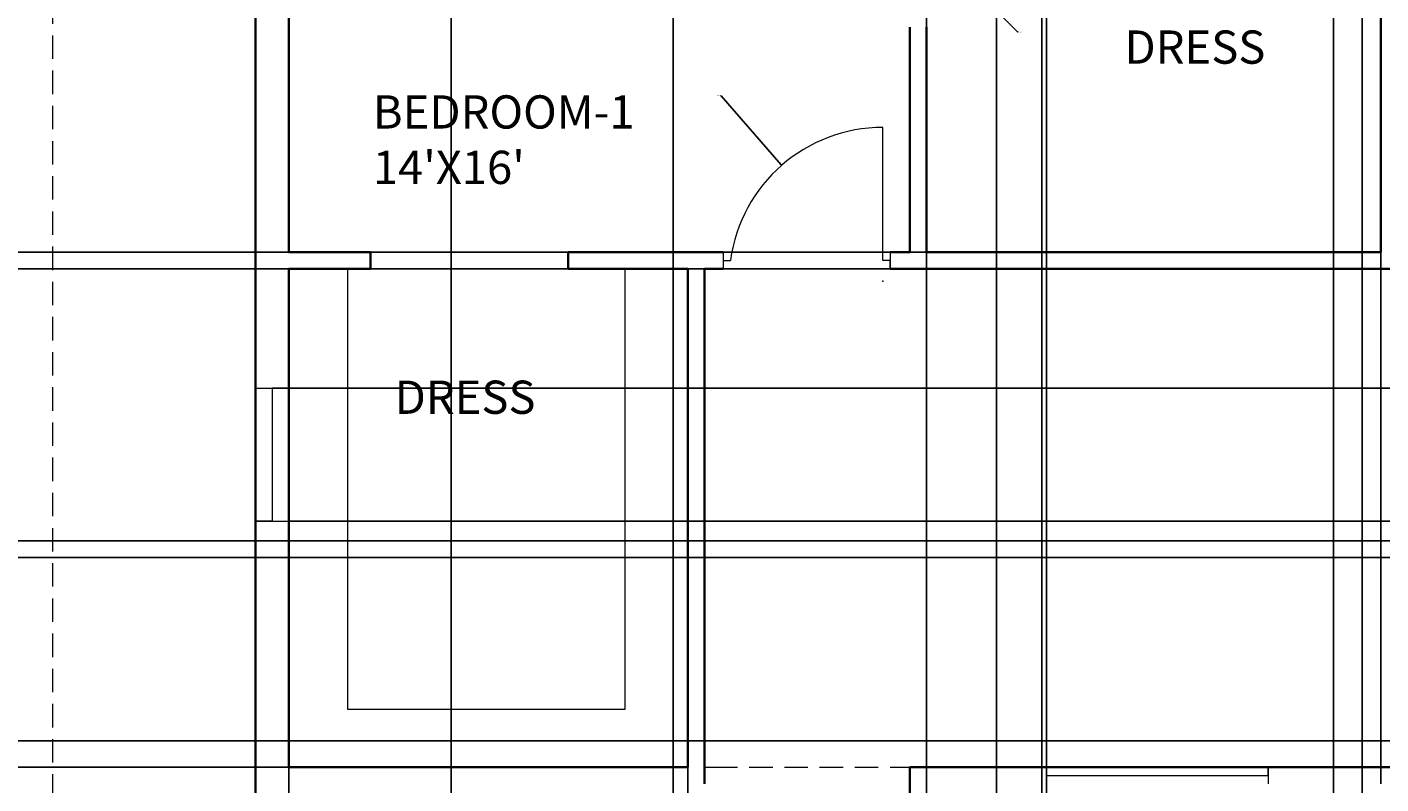
# Model space of a CAD drawing. Units: inches. Extents: x 1770 to 2988, y 1161 to 3221.
# Tile 11 of 44: x 2090 to 2456, y 2032 to 2237. Entities that reach past the tile are written whole.
import ezdxf

# ---------------------------------------------------------------- set-up
doc = ezdxf.new("R2010")
doc.units = ezdxf.units.IN
doc.linetypes.add('DASHED2', pattern=[9.525, 6.35, -3.175])
for name, color, linetype, lineweight in [('A-ANNO-DIMS', 2, 'Continuous', 18), ('A-AREA-IDEN', 7, 'Continuous', 18), ('A-DOOR', 4, 'Continuous', 18), ('A-FLOR-CASE', 8, 'Continuous', 18), ('A-GLAZ', 4, 'Continuous', 18), ('A-ROOF-OVHD', 7, 'DASHED2', 18), ('A-WALL', 7, 'Continuous', 35), ('A-WALL-OVHD', 7, 'DASHED2', 18)]:
    doc.layers.add(name, color=color, linetype=linetype, lineweight=lineweight)
doc.styles.get("Standard").update_dxf_attribs({"font": 'arial.ttf'})
doc.dimstyles.get("Standard").update_dxf_attribs({"dimtxt": 0.18, "dimasz": 0.18, "dimexe": 0.18, "dimexo": 0.0625, "dimgap": 0.09, "dimtad": 0, "dimtih": 1, "dimtoh": 1, "dimdec": 4, "dimzin": 0, "dimdsep": 46, "dimtxsty": 'Standard', "dimcen": 0.09, "dimadec": 0, "dimazin": 0, "dimtfac": 1, "dimtdec": 4, "dimtofl": 0, "dimtmove": 0, "dimatfit": 3, "dimfxl": 1, "dimtolj": 1, "dimtzin": 0, "dimarcsym": 0})

# ---------------------------------------------------------------- blocks, each defined once
blk = doc.blocks.new('WIN-60-COURTYARD')
for p, q in [((0, 4.5), (0, 0)), ((60, 2.25), (60, 4.5)), ((60, 4.5), (60, 0)), ((0, 0), (0, 2.25)), ((0, 2.25), (60, 2.25))]:
    blk.add_line(p, q)
blk = doc.blocks.new('*D63')
at = {"layer": 'A-ANNO-DIMS', "color": 0, "lineweight": -2, "transparency": 16777216}
for p, q in [((2352.17, 1323.59), (2352.17, 2570.7)), ((2352.35, 2570.52), (2401.24, 2570.52)), ((2450.91, 2570.52), (2402.02, 2570.52)), ((2451.09, 1323.59), (2451.09, 2570.7))]:
    blk.add_line(p, q, dxfattribs=at)
at = {"layer": 'A-ANNO-DIMS', "color": 0, "transparency": 16777216}
for points in [[(2352.35, 2570.55), (2352.35, 2570.49), (2352.17, 2570.52)], [(2450.91, 2570.55), (2450.91, 2570.49), (2451.09, 2570.52)]]:
    blk.add_solid(points, dxfattribs=at)
at = {"layer": 'Defpoints', "color": 0, "transparency": 16777216}
for p in [(2451.09, 2570.52), (2352.17, 1323.53), (2451.09, 1323.53)]:
    blk.add_point(p, dxfattribs=at)
at = {"layer": 'A-ANNO-DIMS', "color": 0, "transparency": 16777216, "insert": (2401.63, 2570.52), "char_height": 0.18, "attachment_point": 5}
blk.add_mtext('\\A1;98.93', dxfattribs=at)
blk = doc.blocks.new('*D68')
at = {"layer": 'A-ANNO-DIMS', "color": 0, "lineweight": -2, "transparency": 16777216}
for p, q in [((2333.2, 2031.76), (2333.2, 2570.7)), ((2333.38, 2570.52), (2394.42, 2570.52)), ((2456.02, 2570.52), (2394.98, 2570.52)), ((2456.2, 2031.76), (2456.2, 2570.7))]:
    blk.add_line(p, q, dxfattribs=at)
at = {"layer": 'A-ANNO-DIMS', "color": 0, "transparency": 16777216}
for points in [[(2333.38, 2570.55), (2333.38, 2570.49), (2333.2, 2570.52)], [(2456.02, 2570.55), (2456.02, 2570.49), (2456.2, 2570.52)]]:
    blk.add_solid(points, dxfattribs=at)
at = {"layer": 'Defpoints', "color": 0, "transparency": 16777216}
for p in [(2456.2, 2570.52), (2333.2, 2031.7), (2456.2, 2031.7)]:
    blk.add_point(p, dxfattribs=at)
at = {"layer": 'A-ANNO-DIMS', "color": 0, "transparency": 16777216, "insert": (2394.7, 2570.52), "char_height": 0.18, "attachment_point": 5}
blk.add_mtext('\\A1;123', dxfattribs=at)
blk = doc.blocks.new('*D70')
at = {"layer": 'A-ANNO-DIMS', "color": 0, "lineweight": -2, "transparency": 16777216}
for p, q in [((2160.7, 2171.14), (2160.7, 1165.57)), ((2268.7, 2171.14), (2268.7, 1165.57)), ((2160.88, 1165.75), (2214.42, 1165.75)), ((2268.52, 1165.75), (2214.98, 1165.75))]:
    blk.add_line(p, q, dxfattribs=at)
at = {"layer": 'A-ANNO-DIMS', "color": 0, "transparency": 16777216}
for points in [[(2160.88, 1165.78), (2160.88, 1165.72), (2160.7, 1165.75)], [(2268.52, 1165.78), (2268.52, 1165.72), (2268.7, 1165.75)]]:
    blk.add_solid(points, dxfattribs=at)
at = {"layer": 'Defpoints', "color": 0, "transparency": 16777216}
for p in [(2160.7, 2171.2), (2268.7, 2171.2), (2268.7, 1165.75)]:
    blk.add_point(p, dxfattribs=at)
at = {"layer": 'A-ANNO-DIMS', "color": 0, "transparency": 16777216, "insert": (2214.7, 1165.75), "char_height": 0.18, "attachment_point": 5}
blk.add_mtext('\\A1;108', dxfattribs=at)
blk = doc.blocks.new('*D71')
at = {"layer": 'A-ANNO-DIMS', "color": 0, "lineweight": -2, "transparency": 16777216}
for p, q in [((2160.63, 2171.2), (1907.1, 2171.2)), ((1907.28, 2171.02), (1907.28, 2103.88)), ((1907.28, 2036.38), (1907.28, 2103.52)), ((2160.63, 2036.2), (1907.1, 2036.2))]:
    blk.add_line(p, q, dxfattribs=at)
at = {"layer": 'A-ANNO-DIMS', "color": 0, "transparency": 16777216}
for points in [[(1907.25, 2171.02), (1907.31, 2171.02), (1907.28, 2171.2)], [(1907.25, 2036.38), (1907.31, 2036.38), (1907.28, 2036.2)]]:
    blk.add_solid(points, dxfattribs=at)
at = {"layer": 'Defpoints', "color": 0, "transparency": 16777216}
for p in [(2160.7, 2171.2), (1907.28, 2036.2), (2160.7, 2036.2)]:
    blk.add_point(p, dxfattribs=at)
at = {"layer": 'A-ANNO-DIMS', "color": 0, "transparency": 16777216, "insert": (1907.28, 2103.7), "char_height": 0.18, "attachment_point": 5}
blk.add_mtext('\\A1;135', dxfattribs=at)
blk = doc.blocks.new('*D72')
at = {"layer": 'A-ANNO-DIMS', "color": 0, "lineweight": -2, "transparency": 16777216}
for p, q in [((2456.13, 2267.2), (1907.1, 2267.2)), ((1907.28, 2267.02), (1907.28, 2221.63)), ((1907.28, 2175.88), (1907.28, 2221.27)), ((2456.13, 2175.7), (1907.1, 2175.7))]:
    blk.add_line(p, q, dxfattribs=at)
at = {"layer": 'A-ANNO-DIMS', "color": 0, "transparency": 16777216}
for points in [[(1907.25, 2267.02), (1907.31, 2267.02), (1907.28, 2267.2)], [(1907.25, 2175.88), (1907.31, 2175.88), (1907.28, 2175.7)]]:
    blk.add_solid(points, dxfattribs=at)
at = {"layer": 'Defpoints', "color": 0, "transparency": 16777216}
for p in [(1907.28, 2267.2), (2456.2, 2267.2), (2456.2, 2175.7)]:
    blk.add_point(p, dxfattribs=at)
at = {"layer": 'A-ANNO-DIMS', "color": 0, "transparency": 16777216, "insert": (1907.28, 2221.45), "char_height": 0.18, "attachment_point": 5}
blk.add_mtext('\\A1;91.5', dxfattribs=at)
blk = doc.blocks.new('*D75')
at = {"layer": 'A-ANNO-DIMS', "color": 0, "lineweight": -2, "transparency": 16777216}
for p, q in [((2523.36, 2171.2), (1907.1, 2171.2)), ((1907.28, 2171.02), (1907.28, 2134.56)), ((1907.28, 2097.72), (1907.28, 2134.19)), ((2523.36, 2097.54), (1907.1, 2097.54))]:
    blk.add_line(p, q, dxfattribs=at)
at = {"layer": 'A-ANNO-DIMS', "color": 0, "transparency": 16777216}
for points in [[(1907.25, 2171.02), (1907.31, 2171.02), (1907.28, 2171.2)], [(1907.25, 2097.72), (1907.31, 2097.72), (1907.28, 2097.54)]]:
    blk.add_solid(points, dxfattribs=at)
at = {"layer": 'Defpoints', "color": 0, "transparency": 16777216}
for p in [(2523.42, 2171.2), (1907.28, 2097.54), (2523.42, 2097.54)]:
    blk.add_point(p, dxfattribs=at)
at = {"layer": 'A-ANNO-DIMS', "color": 0, "transparency": 16777216, "insert": (1907.28, 2134.37), "char_height": 0.18, "attachment_point": 5}
blk.add_mtext('\\A1;73.66', dxfattribs=at)
blk = doc.blocks.new('*D79')
at = {"layer": 'A-ANNO-DIMS', "color": 0, "lineweight": -2, "transparency": 16777216}
for p, q in [((2151.7, 1610.26), (2151.7, 2570.7)), ((2151.88, 2570.52), (2177.78, 2570.52)), ((2204.48, 2570.52), (2178.57, 2570.52)), ((2204.66, 1610.26), (2204.66, 2570.7))]:
    blk.add_line(p, q, dxfattribs=at)
at = {"layer": 'A-ANNO-DIMS', "color": 0, "transparency": 16777216}
for points in [[(2151.88, 2570.55), (2151.88, 2570.49), (2151.7, 2570.52)], [(2204.48, 2570.55), (2204.48, 2570.49), (2204.66, 2570.52)]]:
    blk.add_solid(points, dxfattribs=at)
at = {"layer": 'Defpoints', "color": 0, "transparency": 16777216}
for p in [(2204.66, 2570.52), (2151.7, 1610.2), (2204.66, 1610.2)]:
    blk.add_point(p, dxfattribs=at)
at = {"layer": 'A-ANNO-DIMS', "color": 0, "transparency": 16777216, "insert": (2178.18, 2570.52), "char_height": 0.18, "attachment_point": 5}
blk.add_mtext('\\A1;52.96', dxfattribs=at)
blk = doc.blocks.new('*D80')
at = {"layer": 'A-ANNO-DIMS', "color": 0, "lineweight": -2, "transparency": 16777216}
for p, q in [((2264.66, 1610.26), (2264.66, 2570.7)), ((2264.84, 2570.52), (2314.14, 2570.52)), ((2364.23, 2570.52), (2314.93, 2570.52)), ((2364.41, 1610.26), (2364.41, 2570.7))]:
    blk.add_line(p, q, dxfattribs=at)
at = {"layer": 'A-ANNO-DIMS', "color": 0, "transparency": 16777216}
for points in [[(2264.84, 2570.55), (2264.84, 2570.49), (2264.66, 2570.52)], [(2364.23, 2570.55), (2364.23, 2570.49), (2364.41, 2570.52)]]:
    blk.add_solid(points, dxfattribs=at)
at = {"layer": 'Defpoints', "color": 0, "transparency": 16777216}
for p in [(2364.41, 2570.52), (2264.66, 1610.2), (2364.41, 1610.2)]:
    blk.add_point(p, dxfattribs=at)
at = {"layer": 'A-ANNO-DIMS', "color": 0, "transparency": 16777216, "insert": (2314.53, 2570.52), "char_height": 0.18, "attachment_point": 5}
blk.add_mtext('\\A1;99.76', dxfattribs=at)
blk = doc.blocks.new('*D81')
at = {"layer": 'A-ANNO-DIMS', "color": 0, "lineweight": -2, "transparency": 16777216}
for p, q in [((2364.41, 1610.26), (2364.41, 2570.7)), ((2364.59, 2570.52), (2403.51, 2570.52)), ((2443.21, 2570.52), (2404.29, 2570.52)), ((2443.39, 1610.26), (2443.39, 2570.7))]:
    blk.add_line(p, q, dxfattribs=at)
at = {"layer": 'A-ANNO-DIMS', "color": 0, "transparency": 16777216}
for points in [[(2364.59, 2570.55), (2364.59, 2570.49), (2364.41, 2570.52)], [(2443.21, 2570.55), (2443.21, 2570.49), (2443.39, 2570.52)]]:
    blk.add_solid(points, dxfattribs=at)
at = {"layer": 'Defpoints', "color": 0, "transparency": 16777216}
for p in [(2443.39, 2570.52), (2364.41, 1610.2), (2443.39, 1610.2)]:
    blk.add_point(p, dxfattribs=at)
at = {"layer": 'A-ANNO-DIMS', "color": 0, "transparency": 16777216, "insert": (2403.9, 2570.52), "char_height": 0.18, "attachment_point": 5}
blk.add_mtext('\\A1;78.97', dxfattribs=at)
blk = doc.blocks.new('*D82')
at = {"layer": 'A-ANNO-DIMS', "color": 0, "lineweight": -2, "transparency": 16777216}
for p, q in [((2443.39, 1610.26), (2443.39, 2570.7)), ((2443.57, 2570.52), (2486.45, 2570.52)), ((2530.12, 2570.52), (2487.24, 2570.52)), ((2530.3, 1610.26), (2530.3, 2570.7))]:
    blk.add_line(p, q, dxfattribs=at)
at = {"layer": 'A-ANNO-DIMS', "color": 0, "transparency": 16777216}
for points in [[(2443.57, 2570.55), (2443.57, 2570.49), (2443.39, 2570.52)], [(2530.12, 2570.55), (2530.12, 2570.49), (2530.3, 2570.52)]]:
    blk.add_solid(points, dxfattribs=at)
at = {"layer": 'Defpoints', "color": 0, "transparency": 16777216}
for p in [(2530.3, 2570.52), (2443.39, 1610.2), (2530.3, 1610.2)]:
    blk.add_point(p, dxfattribs=at)
at = {"layer": 'A-ANNO-DIMS', "color": 0, "transparency": 16777216, "insert": (2486.85, 2570.52), "char_height": 0.18, "attachment_point": 5}
blk.add_mtext('\\A1;86.92', dxfattribs=at)
blk = doc.blocks.new('*D88')
at = {"layer": 'A-ANNO-DIMS', "color": 0, "lineweight": -2, "transparency": 16777216}
for p, q in [((2523.36, 2093.04), (1907.1, 2093.04)), ((1907.28, 2092.86), (1907.28, 2068.4)), ((1907.28, 2043.57), (1907.28, 2068.04)), ((2523.36, 2043.39), (1907.1, 2043.39))]:
    blk.add_line(p, q, dxfattribs=at)
at = {"layer": 'A-ANNO-DIMS', "color": 0, "transparency": 16777216}
for points in [[(1907.25, 2092.86), (1907.31, 2092.86), (1907.28, 2093.04)], [(1907.25, 2043.57), (1907.31, 2043.57), (1907.28, 2043.39)]]:
    blk.add_solid(points, dxfattribs=at)
at = {"layer": 'Defpoints', "color": 0, "transparency": 16777216}
for p in [(1907.28, 2093.04), (2523.42, 2093.04), (2523.42, 2043.39)]:
    blk.add_point(p, dxfattribs=at)
at = {"layer": 'A-ANNO-DIMS', "color": 0, "transparency": 16777216, "insert": (1907.28, 2068.22), "char_height": 0.18, "attachment_point": 5}
blk.add_mtext('\\A1;49.65', dxfattribs=at)
blk = doc.blocks.new('*D89')
at = {"layer": 'A-ANNO-DIMS', "color": 0, "lineweight": -2, "transparency": 16777216}
for p, q in [((2160.76, 2138.84), (2866.87, 2138.84)), ((2866.69, 2138.66), (2866.69, 2121.02)), ((2866.69, 2103.02), (2866.69, 2120.66)), ((2160.76, 2102.84), (2866.87, 2102.84))]:
    blk.add_line(p, q, dxfattribs=at)
at = {"layer": 'A-ANNO-DIMS', "color": 0, "transparency": 16777216}
for points in [[(2866.66, 2138.66), (2866.72, 2138.66), (2866.69, 2138.84)], [(2866.66, 2103.02), (2866.72, 2103.02), (2866.69, 2102.84)]]:
    blk.add_solid(points, dxfattribs=at)
at = {"layer": 'Defpoints', "color": 0, "transparency": 16777216}
for p in [(2160.7, 2138.84), (2866.69, 2138.84), (2160.7, 2102.84)]:
    blk.add_point(p, dxfattribs=at)
at = {"layer": 'A-ANNO-DIMS', "color": 0, "transparency": 16777216, "insert": (2866.69, 2120.84), "char_height": 0.18, "attachment_point": 5}
blk.add_mtext('\\A1;36', dxfattribs=at)
blk = doc.blocks.new('*D91')
at = {"layer": 'A-ANNO-DIMS', "color": 0, "lineweight": -2, "transparency": 16777216}
for p, q in [((2333.2, 1839.76), (2333.2, 2570.7)), ((2333.38, 2570.52), (2348.97, 2570.52)), ((2365.49, 2570.52), (2349.9, 2570.52)), ((2365.67, 1839.76), (2365.67, 2570.7))]:
    blk.add_line(p, q, dxfattribs=at)
at = {"layer": 'A-ANNO-DIMS', "color": 0, "transparency": 16777216}
for points in [[(2333.38, 2570.55), (2333.38, 2570.49), (2333.2, 2570.52)], [(2365.49, 2570.55), (2365.49, 2570.49), (2365.67, 2570.52)]]:
    blk.add_solid(points, dxfattribs=at)
at = {"layer": 'Defpoints', "color": 0, "transparency": 16777216}
for p in [(2365.67, 2570.52), (2333.2, 1839.7), (2365.67, 1839.7)]:
    blk.add_point(p, dxfattribs=at)
at = {"layer": 'A-ANNO-DIMS', "color": 0, "transparency": 16777216, "insert": (2349.43, 2570.52), "char_height": 0.18, "attachment_point": 5}
blk.add_mtext('\\A1;32.476', dxfattribs=at)
blk = doc.blocks.new('*D110')
at = {"layer": 'A-ANNO-DIMS', "color": 0, "lineweight": -2, "transparency": 16777216}
for p, q in [((2277.46, 2218.01), (2277.64, 2218.01)), ((2277.64, 2218.01), (2293.95, 2199.32)), ((2321.35, 2167.81), (2321.53, 2167.81)), ((2321.44, 2167.72), (2321.44, 2167.9))]:
    blk.add_line(p, q, dxfattribs=at)
at = {"layer": 'A-ANNO-DIMS', "color": 0, "transparency": 16777216}
blk.add_solid([(2293.97, 2199.34), (2293.92, 2199.3), (2294.06, 2199.19)], dxfattribs=at)
at = {"layer": 'Defpoints', "color": 0, "transparency": 16777216}
for p in [(2294.06, 2199.19), (2321.44, 2167.81)]:
    blk.add_point(p, dxfattribs=at)
at = {"layer": 'A-ANNO-DIMS', "color": 0, "transparency": 16777216, "insert": (2276.98, 2218.01), "char_height": 0.18, "attachment_point": 5}
blk.add_mtext('\\A1;R41.64', dxfattribs=at)
blk = doc.blocks.new('*D112')
at = {"layer": 'A-ANNO-DIMS', "color": 0, "lineweight": -2, "transparency": 16777216}
for p, q in [((2331.23, 2262.24), (2331.41, 2262.24)), ((2331.32, 2262.15), (2331.32, 2262.33)), ((2357.84, 2235.3), (2348.02, 2245.28)), ((2358.02, 2235.3), (2357.84, 2235.3))]:
    blk.add_line(p, q, dxfattribs=at)
at = {"layer": 'A-ANNO-DIMS', "color": 0, "transparency": 16777216}
blk.add_solid([(2348.04, 2245.3), (2348, 2245.26), (2347.89, 2245.41)], dxfattribs=at)
at = {"layer": 'Defpoints', "color": 0, "transparency": 16777216}
for p in [(2331.32, 2262.24), (2347.89, 2245.41)]:
    blk.add_point(p, dxfattribs=at)
at = {"layer": 'A-ANNO-DIMS', "color": 0, "transparency": 16777216, "insert": (2358.5, 2235.3), "char_height": 0.18, "attachment_point": 5}
blk.add_mtext('\\A1;R23.63', dxfattribs=at)

msp = doc.modelspace()

# ---------------------------------------------------------------- linework, layer by layer
at = {"layer": 'A-DOOR'}
for p, q in [((2321.4422, 2173.4521), (2321.4422, 2209.4521)), ((2278.1834, 2175.7021), (2278.1834, 2171.2021)), ((2278.1834, 2173.4521), (2280.1834, 2173.4521)), ((2323.4422, 2173.4521), (2321.4422, 2173.4521)), ((2323.4422, 2175.7021), (2323.4422, 2171.2021)), ((2323.4422, 2171.2021), (2323.4422, 2173.4521))]:
    msp.add_line(p, q, dxfattribs=at)
msp.add_arc((2321.4422, 2167.8092), 41.6429, 90, 172.212025, dxfattribs=at)
at = {"layer": 'A-FLOR-CASE'}
for p, q in [((2176.5309, 2171.2021), (2176.5309, 2051.9256)), ((2251.7333, 2051.9256), (2251.7333, 2171.2021)), ((2176.5309, 2051.9256), (2251.7333, 2051.9256))]:
    msp.add_line(p, q, dxfattribs=at)
at = {"layer": 'A-GLAZ'}
for p, q in [((2151.696, 2138.8392), (2160.696, 2138.8392)), ((2160.696, 2138.8392), (2156.196, 2138.8392)), ((2156.196, 2138.8392), (2156.196, 2102.8392)), ((2156.196, 2102.8392), (2151.696, 2102.8392)), ((2151.696, 2102.8392), (2160.696, 2102.8392))]:
    msp.add_line(p, q, dxfattribs=at)
at = {"layer": 'A-ROOF-OVHD'}
msp.add_line((2096.7313, 2405.7876), (2096.7313, 1610.2021), dxfattribs=at)
at = {"layer": 'A-WALL'}
for p, q in [((2151.696, 2376.7021), (2151.696, 1610.2021)), ((2160.696, 2367.7021), (2160.696, 2175.7021)), ((2456.196, 2267.2021), (2456.196, 2175.7021)), ((2328.696, 2236.6179), (2328.696, 2175.7021)), ((2333.196, 2236.6179), (2333.196, 2175.7021)), ((2160.696, 2175.7021), (2182.7786, 2175.7021)), ((2182.7786, 2175.7021), (2182.7786, 2171.2021)), ((2236.2643, 2175.7021), (2236.2643, 2171.2021)), ((2236.2643, 2175.7021), (2278.1834, 2175.7021)), ((2323.4422, 2175.7021), (2328.696, 2175.7021)), ((2333.196, 2175.7021), (2456.196, 2175.7021)), ((2160.696, 2171.2021), (2182.7786, 2171.2021)), ((2160.696, 2171.2021), (2160.696, 2036.2021)), ((2236.2643, 2171.2021), (2268.696, 2171.2021)), ((2268.696, 2171.2021), (2268.696, 2036.2021)), ((2273.196, 2171.2021), (2273.196, 2031.7021)), ((2273.196, 2171.2021), (2278.1834, 2171.2021)), ((2323.4422, 2171.2021), (2468.7272, 2171.2021)), ((2160.696, 2036.2021), (2268.696, 2036.2021)), ((2328.696, 2036.2021), (2328.696, 1835.2021)), ((2328.696, 2036.2021), (2460.696, 2036.2021))]:
    msp.add_line(p, q, dxfattribs=at)
at = {"layer": 'A-WALL-OVHD'}
for p, q in [((2184.4959, 2175.7021), (2236.2643, 2175.7021)), ((2236.2643, 2171.2021), (2182.7786, 2171.2021)), ((2273.196, 2036.2021), (2275.7476, 2036.2021)), ((2275.7476, 2036.2021), (2328.696, 2036.2021))]:
    msp.add_line(p, q, dxfattribs=at)

# ---------------------------------------------------------------- block references
at = {"layer": 'A-GLAZ'}
msp.add_blockref('WIN-60-COURTYARD', (2365.672, 2031.702), dxfattribs=at)

# ---------------------------------------------------------------- texts
at = {"layer": 'A-AREA-IDEN', "char_height": 9, "attachment_point": 1}
for s, width, insert in [('DRESS', 37.691321, (2386.8048, 2235.6986)), ("BEDROOM-1\\P14'X16'", 127.484882, (2183.43, 2218.1375)), ('DRESS', 67.187897, (2189.3188, 2140.8976))]:
    msp.add_mtext_dynamic_manual_height_columns(s, width=width, gutter_width=12.5, heights=[0], dxfattribs=dict(at, insert=insert))

# ---------------------------------------------------------------- dimensions: what is measured, and where the dimension line sits
at = {"layer": 'A-ANNO-DIMS'}
for base, p1, p2, override, picture, middle in [((2204.6568, 2570.5247), (2151.696, 1610.2021), (2204.6568, 1610.2021), {"dimdec": 2, "dimlfac": 1, "dimrnd": 0, "dimzin": 0, "dimdsep": 46, "dimlunit": 2}, '*D79', (2178.1764, 2570.5247)), ((2364.4122, 2570.5247), (2264.6568, 1610.2021), (2364.4122, 1610.2021), {"dimdec": 2, "dimlfac": 1, "dimrnd": 0, "dimzin": 0, "dimdsep": 46, "dimlunit": 2}, '*D80', (2314.5345, 2570.5247)), ((2456.196, 2570.5247), (2333.196, 2031.7021), (2456.196, 2031.7021), {"dimdec": 0, "dimlfac": 1, "dimrnd": 0, "dimzin": 0, "dimdsep": 46, "dimlunit": 2}, '*D68', (2394.696, 2570.5247)), ((2365.672, 2570.5247), (2333.196, 1839.7021), (2365.672, 1839.7021), {"dimdec": 3, "dimlfac": 1, "dimrnd": 0, "dimzin": 0, "dimdsep": 46, "dimlunit": 2}, '*D91', (2349.434, 2570.5247)), ((2451.0947, 2570.5247), (2352.1672, 1323.5288), (2451.0947, 1323.5288), {"dimdec": 2, "dimlfac": 1, "dimrnd": 0, "dimzin": 0, "dimdsep": 46, "dimlunit": 2}, '*D63', (2401.631, 2570.5247)), ((2443.3863, 2570.5247), (2364.4122, 1610.2021), (2443.3863, 1610.2021), {"dimdec": 2, "dimlfac": 1, "dimrnd": 0, "dimzin": 0, "dimdsep": 46, "dimlunit": 2}, '*D81', (2403.8993, 2570.5247)), ((2530.3038, 2570.5247), (2443.3863, 1610.2021), (2530.3038, 1610.2021), {"dimdec": 2, "dimlfac": 1, "dimrnd": 0, "dimzin": 0, "dimdsep": 46, "dimlunit": 2}, '*D82', (2486.8451, 2570.5247)), ((2268.696, 1165.752), (2160.696, 2171.2021), (2268.696, 2171.2021), {"dimdec": 0, "dimlfac": 1, "dimrnd": 0, "dimzin": 0, "dimdsep": 46, "dimlunit": 2}, '*D70', (2214.696, 1165.752))]:
    dim = msp.add_linear_dim(base=base, p1=p1, p2=p2, dimstyle='Standard', override=override, dxfattribs=at)
    dim.commit()
    dim.dimension.update_dxf_attribs({"geometry": picture, "text_midpoint": middle})
for base, p1, p2, override, picture, middle in [((1907.2844, 2267.2021), (2456.196, 2175.7021), (2456.196, 2267.2021), {"dimdec": 1, "dimlfac": 1, "dimrnd": 0, "dimzin": 0, "dimdsep": 46, "dimlunit": 2}, '*D72', (1907.2844, 2221.4521)), ((1907.2844, 2097.5443), (2523.4179, 2171.2021), (2523.4179, 2097.5443), {"dimdec": 2, "dimlfac": 1, "dimrnd": 0, "dimzin": 0, "dimdsep": 46, "dimlunit": 2}, '*D75', (1907.2844, 2134.3732)), ((1907.2844, 2036.2021), (2160.696, 2171.2021), (2160.696, 2036.2021), {"dimdec": 0, "dimlfac": 1, "dimrnd": 0, "dimzin": 0, "dimdsep": 46, "dimlunit": 2}, '*D71', (1907.2844, 2103.7021)), ((2866.6874, 2138.8392), (2160.696, 2102.8392), (2160.696, 2138.8392), {"dimdec": 0, "dimlfac": 1, "dimrnd": 0, "dimzin": 0, "dimdsep": 46, "dimlunit": 2}, '*D89', (2866.6874, 2120.8392)), ((1907.2844, 2093.0443), (2523.4179, 2043.391), (2523.4179, 2093.0443), {"dimdec": 2, "dimlfac": 1, "dimrnd": 0, "dimzin": 0, "dimdsep": 46, "dimlunit": 2}, '*D88', (1907.2844, 2068.2176))]:
    dim = msp.add_linear_dim(base=base, p1=p1, p2=p2, angle=90, dimstyle='Standard', override=override, dxfattribs=at)
    dim.commit()
    dim.dimension.update_dxf_attribs({"geometry": picture, "text_midpoint": middle})
for center, mpoint, picture, middle in [((2331.3164, 2262.2446), (2347.894, 2245.406), '*D112', (2358.5004, 2235.3028)), ((2321.4422, 2167.8092), (2294.064, 2199.187), '*D110', (2276.9776, 2218.0137))]:
    dim = msp.add_radius_dim(center=center, mpoint=mpoint, dimstyle='Standard', override={"dimdec": 2, "dimlfac": 1, "dimrnd": 0, "dimzin": 0, "dimdsep": 46, "dimlunit": 2}, dxfattribs=at)
    dim.commit()
    dim.dimension.update_dxf_attribs({"geometry": picture, "text_midpoint": middle, "dimtype": 164})

doc.saveas('drawing.dxf')
